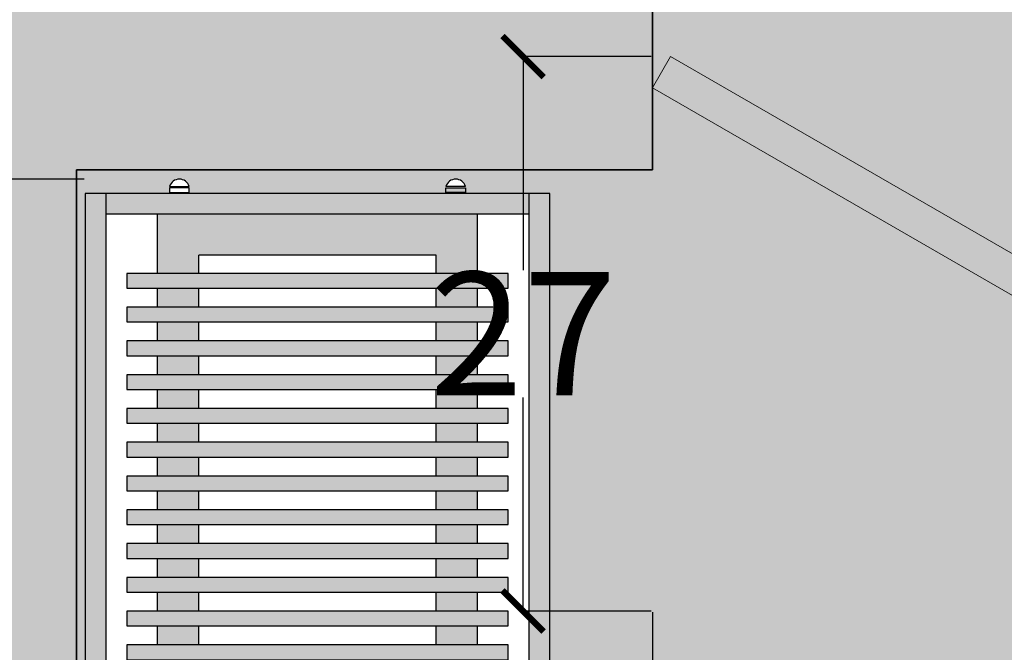
# Model space of a CAD drawing. Units: inches. Extents: x 1704 to 6393, y -157 to 1172.
# Tile 31 of 122: x 2351 to 2398, y 341 to 372. Entities that reach past the tile are written whole.
import ezdxf

# ---------------------------------------------------------------- set-up
doc = ezdxf.new("R2010")
doc.units = ezdxf.units.IN
doc.header["$MEASUREMENT"] = 0
for name, color, linetype, lineweight in [('A-ANNO-DIMS', 7, 'Continuous', 13), ('A-FURN', 8, 'Continuous', 18), ('A-WALL-PATT', 7, 'Continuous', 13), ('DOORS', 160, 'Continuous', 18), ('estofado', 7, 'Continuous', 25), ('WALLS', 7, 'Continuous', 35)]:
    doc.layers.add(name, color=color, linetype=linetype, lineweight=lineweight)
doc.layers.add('A-FLOR-PATT', color=7, linetype='Continuous', lineweight=13, true_color=0xf2f2f2)
doc.layers.add('MOBIL', color=7, linetype='Continuous')
doc.styles.get("Standard").update_dxf_attribs({"font": 'arial.ttf'})
doc.dimstyles.get("Standard").update_dxf_attribs({"dimtxt": 6, "dimasz": 2, "dimexe": 0.18, "dimexo": 0.0625, "dimgap": 0.09, "dimtad": 0, "dimtih": 1, "dimtoh": 1, "dimdec": 1, "dimzin": 0, "dimdsep": 46, "dimlunit": 3, "dimtxsty": 'Standard', "dimblk": 'ARCHTICK', "dimcen": 0.09, "dimadec": 0, "dimazin": 0, "dimtfac": 1, "dimtdec": 1, "dimtofl": 0, "dimtmove": 0, "dimatfit": 3, "dimfxl": 1, "dimtolj": 1, "dimtzin": 0, "dimarcsym": 0})

# ---------------------------------------------------------------- blocks, each defined once
blk = doc.blocks.new('Door - Left Hung 36 in.')
blk.add_lwpolyline([(0.75, -1.299), (0, 0), (31.177, 18), (31.927, 16.701)], close=True)
blk.add_arc((0, 0), 36, 0, 37.3101)
blk = doc.blocks.new('Aparador Aido WV')
at = {"layer": 'MOBIL'}
h = blk.add_hatch(color=256, dxfattribs=at)
h.set_gradient(color1=(226, 228, 228), one_color=1, tint=1, name='CYLINDER')
h.paths.add_polyline_path([(0.9, -0.02), (0.9, 0), (-0.9, 0), (-0.9, -0.02)])
h = blk.add_hatch(color=256, dxfattribs=at)
h.set_gradient(color1=(226, 228, 228), one_color=1, tint=1)
h.paths.add_polyline_path([(0.9, -0.02), (0.88, -0.02), (0.88, -0.43), (0.9, -0.43)])
h = blk.add_hatch(color=256, dxfattribs=at)
h.set_gradient(color1=(106, 79, 62), color2=(55, 41, 32), one_color=1, tint=0.17)
h.paths.add_polyline_path([(0.44785, -0.04017), (0.44785, -0.40983), (0.46222, -0.40983), (0.46222, -0.04017)])
h = blk.add_hatch(color=256, dxfattribs=at)
h.set_gradient(color1=(106, 79, 62), color2=(55, 41, 32), one_color=1, tint=0.17)
h.paths.add_polyline_path([(0.4806, -0.04017), (0.4806, -0.40983), (0.49497, -0.40983), (0.49497, -0.04017)])
h = blk.add_hatch(color=256, dxfattribs=at)
h.set_gradient(color1=(106, 79, 62), color2=(55, 41, 32), one_color=1, tint=0.17)
h.paths.add_polyline_path([(0.51335, -0.04017), (0.51335, -0.40983), (0.52772, -0.40983), (0.52772, -0.04017)])
h = blk.add_hatch(color=256, dxfattribs=at)
h.set_gradient(color1=(106, 79, 62), color2=(55, 41, 32), one_color=1, tint=0.17)
h.paths.add_polyline_path([(0.54611, -0.04017), (0.54611, -0.40983), (0.56047, -0.40983), (0.56047, -0.04017)])
h = blk.add_hatch(color=256, dxfattribs=at)
h.set_gradient(color1=(106, 79, 62), color2=(55, 41, 32), one_color=1, tint=0.17)
h.paths.add_polyline_path([(0.57886, -0.04017), (0.57886, -0.40983), (0.59322, -0.40983), (0.59322, -0.04017)])
h = blk.add_hatch(color=256, dxfattribs=at)
h.set_gradient(color1=(106, 79, 62), color2=(55, 41, 32), one_color=1, tint=0.17)
h.paths.add_polyline_path([(0.61161, -0.04017), (0.61161, -0.40983), (0.62597, -0.40983), (0.62597, -0.04017)])
h = blk.add_hatch(color=256, dxfattribs=at)
h.set_gradient(color1=(106, 79, 62), color2=(55, 41, 32), one_color=1, tint=0.17)
h.paths.add_polyline_path([(0.64436, -0.04017), (0.64436, -0.40983), (0.65873, -0.40983), (0.65873, -0.04017)])
h = blk.add_hatch(color=256, dxfattribs=at)
h.set_gradient(color1=(106, 79, 62), color2=(55, 41, 32), one_color=1, tint=0.17)
h.paths.add_polyline_path([(0.67711, -0.04017), (0.67711, -0.40983), (0.69148, -0.40983), (0.69148, -0.04017)])
h = blk.add_hatch(color=256, dxfattribs=at)
h.set_gradient(color1=(106, 79, 62), color2=(55, 41, 32), one_color=1, tint=0.17)
h.paths.add_polyline_path([(0.70986, -0.04017), (0.70986, -0.40983), (0.72423, -0.40983), (0.72423, -0.04017)])
h = blk.add_hatch(color=256, dxfattribs=at)
h.set_gradient(color1=(106, 79, 62), color2=(55, 41, 32), one_color=1, tint=0.17)
h.paths.add_polyline_path([(0.74262, -0.04017), (0.74262, -0.40983), (0.75698, -0.40983), (0.75698, -0.04017)])
h = blk.add_hatch(color=256, dxfattribs=at)
h.set_gradient(color1=(106, 79, 62), color2=(55, 41, 32), one_color=1, tint=0.17)
h.paths.add_polyline_path([(0.77537, -0.04017), (0.77537, -0.40983), (0.78973, -0.40983), (0.78973, -0.04017)])
h = blk.add_hatch(color=256, dxfattribs=at)
h.set_gradient(color1=(106, 79, 62), color2=(55, 41, 32), one_color=1, tint=0.17)
h.paths.add_polyline_path([(0.80812, -0.04017), (0.80812, -0.40983), (0.82248, -0.40983), (0.82248, -0.04017)])
h = blk.add_hatch(color=256, dxfattribs=at)
h.set_gradient(color1=(106, 79, 62), color2=(157, 117, 92), one_color=1, tint=0.49)
h.paths.add_polyline_path([(0.4806, -0.07), (0.46222, -0.07), (0.46222, -0.11), (0.4806, -0.11)])
h = blk.add_hatch(color=256, dxfattribs=at)
h.set_gradient(color1=(106, 79, 62), color2=(157, 117, 92), one_color=1, tint=0.49)
h.paths.add_polyline_path([(0.51335, -0.07), (0.49497, -0.07), (0.49497, -0.11), (0.51335, -0.11)])
h = blk.add_hatch(color=256, dxfattribs=at)
h.set_gradient(color1=(106, 79, 62), color2=(157, 117, 92), one_color=1, tint=0.49)
h.paths.add_polyline_path([(0.52772, -0.11), (0.54611, -0.11), (0.54611, -0.07), (0.52772, -0.07)])
h = blk.add_hatch(color=256, dxfattribs=at)
h.set_gradient(color1=(106, 79, 62), color2=(157, 117, 92), one_color=1, tint=0.49)
h.paths.add_polyline_path([(0.57886, -0.07), (0.56047, -0.07), (0.56047, -0.11), (0.57886, -0.11)])
h = blk.add_hatch(color=256, dxfattribs=at)
h.set_gradient(color1=(106, 79, 62), color2=(157, 117, 92), one_color=1, tint=0.49)
h.paths.add_polyline_path([(0.61161, -0.07), (0.59322, -0.07), (0.59322, -0.11), (0.61161, -0.11)])
h = blk.add_hatch(color=256, dxfattribs=at)
h.set_gradient(color1=(106, 79, 62), color2=(157, 117, 92), one_color=1, tint=0.49)
h.paths.add_polyline_path([(0.64436, -0.07), (0.62597, -0.07), (0.62597, -0.11), (0.64436, -0.11)])
h = blk.add_hatch(color=256, dxfattribs=at)
h.set_gradient(color1=(106, 79, 62), color2=(157, 117, 92), one_color=1, tint=0.49)
h.paths.add_polyline_path([(0.67711, -0.07), (0.65873, -0.07), (0.65873, -0.11), (0.67711, -0.11)])
h = blk.add_hatch(color=256, dxfattribs=at)
h.set_gradient(color1=(106, 79, 62), color2=(157, 117, 92), one_color=1, tint=0.49)
h.paths.add_polyline_path([(0.70986, -0.07), (0.69148, -0.07), (0.69148, -0.11), (0.70986, -0.11)])
h = blk.add_hatch(color=256, dxfattribs=at)
h.set_gradient(color1=(106, 79, 62), color2=(157, 117, 92), one_color=1, tint=0.49)
h.paths.add_polyline_path([(0.74262, -0.07), (0.72423, -0.07), (0.72423, -0.11), (0.74262, -0.11)])
h = blk.add_hatch(color=256, dxfattribs=at)
h.set_gradient(color1=(106, 79, 62), color2=(157, 117, 92), one_color=1, tint=0.49)
h.paths.add_polyline_path([(0.77537, -0.07), (0.75698, -0.07), (0.75698, -0.11), (0.77537, -0.11)])
h = blk.add_hatch(color=256, dxfattribs=at)
h.set_gradient(color1=(106, 79, 62), color2=(157, 117, 92), one_color=1, tint=0.49)
h.paths.add_polyline_path([(0.80812, -0.07), (0.78973, -0.07), (0.78973, -0.11), (0.80812, -0.11)])
h = blk.add_hatch(color=256, dxfattribs=at)
h.set_gradient(color1=(106, 79, 62), color2=(157, 117, 92), one_color=1, tint=0.49)
h.paths.add_polyline_path([(0.88, -0.07), (0.82248, -0.07), (0.82248, -0.11), (0.84, -0.11), (0.84, -0.34), (0.82248, -0.34), (0.82248, -0.38), (0.88, -0.38)])
h = blk.add_hatch(color=256, dxfattribs=at)
h.set_gradient(color1=(106, 79, 62), color2=(157, 117, 92), one_color=1, tint=0.49)
h.paths.add_polyline_path([(0.4806, -0.34), (0.46222, -0.34), (0.46222, -0.38), (0.4806, -0.38)])
h = blk.add_hatch(color=256, dxfattribs=at)
h.set_gradient(color1=(106, 79, 62), color2=(157, 117, 92), one_color=1, tint=0.49)
h.paths.add_polyline_path([(0.51335, -0.34), (0.49497, -0.34), (0.49497, -0.38), (0.51335, -0.38)])
h = blk.add_hatch(color=256, dxfattribs=at)
h.set_gradient(color1=(106, 79, 62), color2=(157, 117, 92), one_color=1, tint=0.49)
h.paths.add_polyline_path([(0.54611, -0.34), (0.52772, -0.34), (0.52772, -0.38), (0.54611, -0.38)])
h = blk.add_hatch(color=256, dxfattribs=at)
h.set_gradient(color1=(106, 79, 62), color2=(157, 117, 92), one_color=1, tint=0.49)
h.paths.add_polyline_path([(0.57886, -0.34), (0.56047, -0.34), (0.56047, -0.38), (0.57886, -0.38)])
h = blk.add_hatch(color=256, dxfattribs=at)
h.set_gradient(color1=(106, 79, 62), color2=(157, 117, 92), one_color=1, tint=0.49)
h.paths.add_polyline_path([(0.61161, -0.34), (0.59322, -0.34), (0.59322, -0.38), (0.61161, -0.38)])
h = blk.add_hatch(color=256, dxfattribs=at)
h.set_gradient(color1=(106, 79, 62), color2=(157, 117, 92), one_color=1, tint=0.49)
h.paths.add_polyline_path([(0.64436, -0.34), (0.62597, -0.34), (0.62597, -0.38), (0.64436, -0.38)])
h = blk.add_hatch(color=256, dxfattribs=at)
h.set_gradient(color1=(106, 79, 62), color2=(157, 117, 92), one_color=1, tint=0.49)
h.paths.add_polyline_path([(0.67711, -0.34), (0.65873, -0.34), (0.65873, -0.38), (0.67711, -0.38)])
h = blk.add_hatch(color=256, dxfattribs=at)
h.set_gradient(color1=(106, 79, 62), color2=(157, 117, 92), one_color=1, tint=0.49)
h.paths.add_polyline_path([(0.70986, -0.34), (0.69148, -0.34), (0.69148, -0.38), (0.70986, -0.38)])
h = blk.add_hatch(color=256, dxfattribs=at)
h.set_gradient(color1=(106, 79, 62), color2=(157, 117, 92), one_color=1, tint=0.49)
h.paths.add_polyline_path([(0.74262, -0.34), (0.72423, -0.34), (0.72423, -0.38), (0.74262, -0.38)])
h = blk.add_hatch(color=256, dxfattribs=at)
h.set_gradient(color1=(106, 79, 62), color2=(157, 117, 92), one_color=1, tint=0.49)
h.paths.add_polyline_path([(0.77537, -0.34), (0.75698, -0.34), (0.75698, -0.38), (0.77537, -0.38)])
h = blk.add_hatch(color=256, dxfattribs=at)
h.set_gradient(color1=(106, 79, 62), color2=(157, 117, 92), one_color=1, tint=0.49)
h.paths.add_polyline_path([(0.80812, -0.34), (0.78973, -0.34), (0.78973, -0.38), (0.80812, -0.38)])
h = blk.add_hatch(color=256, dxfattribs=at)
h.set_gradient(color1=(226, 228, 228), one_color=1, tint=1, name='CYLINDER')
h.paths.add_polyline_path([(0.9, -0.45), (0.9, -0.43), (-0.9, -0.43), (-0.9, -0.45)])
at = {"layer": 'estofado', "ltscale": 0.5}
for p, q in [((0.46222, -0.07), (0.4806, -0.07)), ((0.49497, -0.07), (0.51335, -0.07)), ((0.52772, -0.07), (0.54611, -0.07)), ((0.56047, -0.07), (0.57886, -0.07)), ((0.59322, -0.07), (0.61161, -0.07)), ((0.62597, -0.07), (0.64436, -0.07)), ((0.65873, -0.07), (0.67711, -0.07)), ((0.69148, -0.07), (0.70986, -0.07)), ((0.72423, -0.07), (0.74262, -0.07)), ((0.75698, -0.07), (0.77537, -0.07)), ((0.78973, -0.07), (0.80812, -0.07)), ((0.82248, -0.07), (0.88, -0.07)), ((0.90671, -0.0817), (0.90671, -0.10055)), ((0.46222, -0.11), (0.4806, -0.11)), ((0.49497, -0.11), (0.51335, -0.11)), ((0.52772, -0.11), (0.54611, -0.11)), ((0.56047, -0.11), (0.57886, -0.11)), ((0.59322, -0.11), (0.61161, -0.11)), ((0.62597, -0.11), (0.64436, -0.11)), ((0.65873, -0.11), (0.67711, -0.11)), ((0.69148, -0.11), (0.70986, -0.11)), ((0.72423, -0.11), (0.74262, -0.11)), ((0.75698, -0.11), (0.77537, -0.11)), ((0.78973, -0.11), (0.80812, -0.11)), ((0.82248, -0.11), (0.84, -0.11)), ((0.84, -0.34), (0.84, -0.11)), ((0.46222, -0.34), (0.4806, -0.34)), ((0.49497, -0.34), (0.51335, -0.34)), ((0.52772, -0.34), (0.54611, -0.34)), ((0.56047, -0.34), (0.57886, -0.34)), ((0.59322, -0.34), (0.61161, -0.34)), ((0.62597, -0.34), (0.64436, -0.34)), ((0.65873, -0.34), (0.67711, -0.34)), ((0.69148, -0.34), (0.70986, -0.34)), ((0.72423, -0.34), (0.74262, -0.34)), ((0.75698, -0.34), (0.77537, -0.34)), ((0.78973, -0.34), (0.80812, -0.34)), ((0.82248, -0.34), (0.84, -0.34)), ((0.90671, -0.3683), (0.90671, -0.34945)), ((0.46222, -0.38), (0.4806, -0.38)), ((0.49497, -0.38), (0.51335, -0.38)), ((0.52772, -0.38), (0.54611, -0.38)), ((0.56047, -0.38), (0.57886, -0.38)), ((0.59322, -0.38), (0.61161, -0.38)), ((0.62597, -0.38), (0.64436, -0.38)), ((0.65873, -0.38), (0.67711, -0.38)), ((0.69148, -0.38), (0.70986, -0.38)), ((0.72423, -0.38), (0.74262, -0.38)), ((0.75698, -0.38), (0.77537, -0.38)), ((0.78973, -0.38), (0.80812, -0.38)), ((0.82248, -0.38), (0.88, -0.38))]:
    blk.add_line(p, q, dxfattribs=at)
for points in [[(0.44785, -0.04017), (0.44785, -0.40983), (0.46222, -0.40983), (0.46222, -0.04017)], [(0.4806, -0.04017), (0.4806, -0.40983), (0.49497, -0.40983), (0.49497, -0.04017)], [(0.51335, -0.04017), (0.51335, -0.40983), (0.52772, -0.40983), (0.52772, -0.04017)], [(0.54611, -0.04017), (0.54611, -0.40983), (0.56047, -0.40983), (0.56047, -0.04017)], [(0.57886, -0.04017), (0.57886, -0.40983), (0.59322, -0.40983), (0.59322, -0.04017)], [(0.61161, -0.04017), (0.61161, -0.40983), (0.62597, -0.40983), (0.62597, -0.04017)], [(0.64436, -0.04017), (0.64436, -0.40983), (0.65873, -0.40983), (0.65873, -0.04017)], [(0.67711, -0.04017), (0.67711, -0.40983), (0.69148, -0.40983), (0.69148, -0.04017)], [(0.70986, -0.04017), (0.70986, -0.40983), (0.72423, -0.40983), (0.72423, -0.04017)], [(0.74262, -0.04017), (0.74262, -0.40983), (0.75698, -0.40983), (0.75698, -0.04017)], [(0.77537, -0.04017), (0.77537, -0.40983), (0.78973, -0.40983), (0.78973, -0.04017)], [(0.80812, -0.04017), (0.80812, -0.40983), (0.82248, -0.40983), (0.82248, -0.04017)], [(0.90536, -0.0817), (0.90086, -0.0817), (0.90086, -0.10055), (0.90536, -0.10055)], [(0.90536, -0.3683), (0.90086, -0.3683), (0.90086, -0.34945), (0.90536, -0.34945)]]:
    blk.add_lwpolyline(points, close=True, dxfattribs=at)
for centre in [(0.90401, -0.09113), (0.90401, -0.35887)]:
    blk.add_arc(centre, 0.0098, 285.98491, 74.01509, dxfattribs=at)
at = {"layer": 'MOBIL'}
for p, q in [((0.9, -0.02), (-0.9, -0.02)), ((0.88, -0.43), (0.88, -0.02)), ((-0.9, -0.43), (0.9, -0.43))]:
    blk.add_line(p, q, dxfattribs=at)
blk.add_lwpolyline([(-0.9, -0.45), (0.9, -0.45), (0.9, 0), (-0.9, 0)], close=True, dxfattribs=at)
blk = doc.blocks.new('_ArchTick')
at = {"color": 0, "linetype": 'ByBlock', "const_width": 0.15}
blk.add_lwpolyline([(-0.5, -0.5), (0.5, 0.5)], dxfattribs=at)
blk = doc.blocks.new('*D30')
at = {"layer": 'A-ANNO-DIMS', "color": 0, "lineweight": -2, "transparency": 16777216}
for p, q in [((2381.349, 342.693), (2381.349, 336.276)), ((2423.349, 342.693), (2423.349, 336.276)), ((2381.349, 336.456), (2384.404, 336.456)), ((2423.349, 336.456), (2420.293, 336.456))]:
    blk.add_line(p, q, dxfattribs=at)
at = {"layer": 'Defpoints', "color": 0, "lineweight": -3, "transparency": 16777216}
for p in [(2381.349, 342.756), (2423.349, 342.756), (2423.349, 336.456)]:
    blk.add_point(p, dxfattribs=at)
at = {"layer": 'A-ANNO-DIMS', "color": 0, "lineweight": -2, "transparency": 16777216, "xscale": 2, "yscale": 2, "zscale": 2, "rotation": 180}
blk.add_blockref('_ArchTick', (2381.349, 336.456), dxfattribs=at)
at = {"layer": 'A-ANNO-DIMS', "color": 0, "lineweight": -2, "transparency": 16777216, "xscale": 2, "yscale": 2, "zscale": 2}
blk.add_blockref('_ArchTick', (2423.349, 336.456), dxfattribs=at)
at = {"layer": 'A-ANNO-DIMS', "color": 0, "transparency": 16777216, "insert": (2402.349, 336.456), "char_height": 6, "attachment_point": 5}
blk.add_mtext('\\A1;DOOR 42', dxfattribs=at)
blk = doc.blocks.new('*D31')
at = {"layer": 'A-ANNO-DIMS', "color": 0, "lineweight": -2, "transparency": 16777216}
for p, q in [((2381.286, 369.729), (2374.869, 369.729)), ((2375.049, 369.729), (2375.049, 359.344)), ((2375.049, 342.756), (2375.049, 353.14)), ((2381.286, 342.756), (2374.869, 342.756))]:
    blk.add_line(p, q, dxfattribs=at)
at = {"layer": 'Defpoints', "color": 0, "lineweight": -3, "transparency": 16777216}
for p in [(2381.349, 369.729), (2375.049, 342.756), (2381.349, 342.756)]:
    blk.add_point(p, dxfattribs=at)
at = {"layer": 'A-ANNO-DIMS', "color": 0, "lineweight": -2, "transparency": 16777216, "xscale": 2, "yscale": 2, "zscale": 2}
for p, rotation in [((2375.049, 369.729), 90), ((2375.049, 342.756), 270)]:
    blk.add_blockref('_ArchTick', p, dxfattribs=dict(at, rotation=rotation))
at = {"layer": 'A-ANNO-DIMS', "color": 0, "transparency": 16777216, "insert": (2375.049, 356.242), "char_height": 6, "attachment_point": 5}
blk.add_mtext('\\A1;27', dxfattribs=at)
blk = doc.blocks.new('*D68')
at = {"layer": 'A-ANNO-DIMS', "color": 0, "lineweight": -2, "transparency": 16777216}
for p, q in [((2353.706, 363.767), (2339.834, 363.767)), ((2340.014, 363.767), (2340.014, 321.111)), ((2340.014, 272.066), (2340.014, 314.722)), ((2353.706, 272.066), (2339.834, 272.066))]:
    blk.add_line(p, q, dxfattribs=at)
at = {"layer": 'Defpoints', "color": 0, "lineweight": -3, "transparency": 16777216}
for p in [(2340.014, 363.767), (2353.769, 363.767), (2353.769, 272.066)]:
    blk.add_point(p, dxfattribs=at)
at = {"layer": 'A-ANNO-DIMS', "color": 0, "lineweight": -2, "transparency": 16777216, "xscale": 2, "yscale": 2, "zscale": 2}
for p, rotation in [((2340.014, 363.767), 90), ((2340.014, 272.066), 270)]:
    blk.add_blockref('_ArchTick', p, dxfattribs=dict(at, rotation=rotation))
at = {"layer": 'A-ANNO-DIMS', "color": 0, "transparency": 16777216, "insert": (2340.014, 317.916), "char_height": 6, "attachment_point": 5}
blk.add_mtext('\\A1;SIDEBOARD 92', dxfattribs=at)
blk = doc.blocks.new('*D93')
at = {"layer": 'A-ANNO-DIMS', "color": 0, "lineweight": -2, "transparency": 16777216}
for p, q in [((2605.286, 895.213), (1829.698, 895.213)), ((1829.878, 895.213), (1829.878, 495.866)), ((1829.878, 90.213), (1829.878, 489.56)), ((2605.286, 90.213), (1829.698, 90.213))]:
    blk.add_line(p, q, dxfattribs=at)
at = {"layer": 'Defpoints', "color": 0, "lineweight": -3, "transparency": 16777216}
for p in [(2605.349, 895.213), (1829.878, 90.213), (2605.349, 90.213)]:
    blk.add_point(p, dxfattribs=at)
at = {"layer": 'A-ANNO-DIMS', "color": 0, "lineweight": -2, "transparency": 16777216, "xscale": 2, "yscale": 2, "zscale": 2}
for p, rotation in [((1829.878, 895.213), 90), ((1829.878, 90.213), 270)]:
    blk.add_blockref('_ArchTick', p, dxfattribs=dict(at, rotation=rotation))
at = {"layer": 'A-ANNO-DIMS', "color": 0, "transparency": 16777216, "insert": (1829.878, 492.713), "char_height": 6, "attachment_point": 5}
blk.add_mtext('\\A1;805', dxfattribs=at)

msp = doc.modelspace()

# ---------------------------------------------------------------- hatches: boundary and pattern name
at = {"layer": 'A-FLOR-PATT', "transparency": 33554528}
h = msp.add_hatch(color=256, dxfattribs=at)
h.dxf.hatch_style = 1
h.paths.add_polyline_path([(2325.349, 863.213), (2325.349, 887.213), (2263.349, 887.213), (2167.349, 887.213), (2081.349, 887.213), (2081.349, 719.213), (2277.349, 719.213), (2277.349, 711.213), (2277.349, 372.213), (2349.349, 372.213), (2381.349, 372.213), (2381.349, 364.213), (2353.349, 364.213), (2353.349, 270.213), (2381.349, 270.213), (2381.349, 266.213), (2357.349, 266.213), (2357.349, 98.213), (2381.349, 98.213), (2385.181, 98.213), (2386.482, 98.213), (2424.215, 98.213), (2425.516, 98.213), (2429.349, 98.213), (2597.349, 98.213), (2597.349, 146.213), (2597.349, 218.213), (2597.349, 266.213), (2423.349, 266.213), (2423.349, 270.213), (2473.349, 270.213), (2473.349, 294.213), (2477.349, 294.213), (2477.349, 270.213), (2547.349, 270.213), (2547.349, 364.213), (2477.349, 364.213), (2477.349, 318.213), (2473.349, 318.213), (2473.349, 364.213), (2423.349, 364.213), (2423.349, 372.213), (2469.349, 372.213), (2469.349, 459.213), (2469.349, 538.213), (2350.349, 538.213), (2350.349, 565.713), (2358.349, 565.713), (2358.349, 545.213), (2420.349, 545.213), (2420.349, 610.213), (2358.349, 610.213), (2358.349, 589.713), (2350.349, 589.713), (2350.349, 615.213), (2425.349, 615.213), (2425.349, 607.213), (2425.349, 546.213), (2469.349, 546.213), (2514.349, 546.213), (2514.349, 607.213), (2449.349, 607.213), (2449.349, 615.213), (2451.738, 615.213), (2451.738, 659.213), (2427.738, 659.213), (2427.738, 665.213), (2367.738, 665.213), (2367.738, 667.213), (2367.738, 711.213), (2325.349, 711.213), (2325.349, 719.213), (2325.349, 755.213), (2325.349, 763.213)])
h.paths.add_polyline_path([(2233.858, 822.533, -0.187247), (2233.858, 809.14), (2231.697, 808.804, 0.084893), (2233.131, 814.486), (2230.424, 814.486, -0.104258), (2228.553, 808.313), (2217.751, 807.156, -0.222222), (2217.751, 824.517), (2228.553, 823.359, -0.104258), (2230.424, 817.186), (2233.131, 817.186, 0.084893), (2231.697, 822.868)], flags=16)
h.paths.add_polyline_path([(2213.621, 833.197), (2213.621, 798.475), (2156.048, 798.475), (2156.048, 833.197)], flags=16)
h.paths.add_polyline_path([(2203.932, 848.099), (2205.089, 837.296, -0.222222), (2187.728, 837.296), (2188.885, 848.099, -0.104258), (2195.058, 849.969), (2195.058, 852.676, 0.084893), (2189.377, 851.242), (2189.712, 853.404, -0.187247), (2203.105, 853.404), (2203.44, 851.242, 0.084893), (2197.759, 852.676), (2197.759, 849.969, -0.104258)], flags=16)
h.paths.add_polyline_path([(2181.941, 837.296, -0.222222), (2164.58, 837.296), (2165.737, 848.099, -0.104258), (2171.91, 849.969), (2171.91, 852.676, 0.084893), (2166.229, 851.242), (2166.564, 853.404, -0.187247), (2179.957, 853.404), (2180.292, 851.242, 0.084893), (2174.611, 852.676), (2174.611, 849.969, -0.104258), (2180.784, 848.099)], flags=16)
h.paths.add_polyline_path([(2205.089, 794.376), (2203.932, 783.574, -0.104258), (2197.759, 781.703), (2197.759, 778.996, 0.084893), (2203.44, 780.43), (2203.105, 778.269, -0.187247), (2189.712, 778.269), (2189.377, 780.43, 0.084893), (2195.058, 778.996), (2195.058, 781.703, -0.104258), (2188.885, 783.574), (2187.728, 794.376, -0.222222)], flags=16)
h.paths.add_polyline_path([(2181.941, 794.376), (2180.784, 783.574, -0.104258), (2174.611, 781.703), (2174.611, 778.996, 0.084893), (2180.292, 780.43), (2179.957, 778.269, -0.187247), (2166.564, 778.269), (2166.229, 780.43, 0.084893), (2171.91, 778.996), (2171.91, 781.703, -0.104258), (2165.737, 783.574), (2164.58, 794.376, -0.222222)], flags=16)
h.paths.add_polyline_path([(2151.918, 807.156), (2141.116, 808.313, -0.104258), (2139.245, 814.486), (2136.539, 814.486, 0.084893), (2137.972, 808.804), (2135.811, 809.14, -0.187247), (2135.811, 822.533), (2137.972, 822.868, 0.084893), (2136.539, 817.186), (2139.245, 817.186, -0.104258), (2141.116, 823.359), (2151.918, 824.517, -0.222222)], flags=16)
h.paths.add_polyline_path([(2357.868, 363.41), (2358.814, 363.41, 0.75376)], flags=16)
h.paths.add_polyline_path([(2372.241, 363.117), (2372.248, 363.117), (2372.248, 363.343), (2371.302, 363.343), (2371.302, 363.139, -1.360391)], flags=16)
h.paths.add_polyline_path([(2371.309, 272.716), (2371.302, 272.716), (2371.302, 272.49), (2372.248, 272.49), (2372.248, 272.693, -1.360391)], flags=16)
h.paths.add_polyline_path([(2357.875, 272.716), (2357.868, 272.716), (2357.868, 272.49), (2358.814, 272.49), (2358.814, 272.693, -1.360391)], flags=16)
h.paths.add_polyline_path([(2353.769, 363.074), (2376.347, 363.074), (2376.347, 272.759), (2353.769, 272.759)], flags=16)
h.paths.add_polyline_path([(2354.772, 362.07), (2375.344, 362.07), (2375.344, 273.762), (2354.772, 273.762)], flags=0)
h.paths.add_polyline_path([(2357.868, 363.343), (2358.814, 363.343), (2358.814, 363.117), (2357.868, 363.117)], flags=16)
h.paths.add_polyline_path([(2359.288, 359.184), (2359.288, 360.063), (2370.828, 360.063), (2370.828, 359.184), (2374.332, 359.184), (2374.332, 358.464), (2372.835, 358.464), (2372.835, 357.541), (2374.332, 357.541), (2374.332, 356.82), (2372.835, 356.82), (2372.835, 355.898), (2374.332, 355.898), (2374.332, 355.177), (2372.835, 355.177), (2372.835, 354.254), (2374.332, 354.254), (2374.332, 353.534), (2372.835, 353.534), (2372.835, 352.611), (2374.332, 352.611), (2374.332, 351.89), (2372.835, 351.89), (2372.835, 350.968), (2374.332, 350.968), (2374.332, 350.247), (2372.835, 350.247), (2372.835, 349.324), (2374.332, 349.324), (2374.332, 348.604), (2372.835, 348.604), (2372.835, 347.681), (2374.332, 347.681), (2374.332, 346.96), (2372.835, 346.96), (2372.835, 346.038), (2374.332, 346.038), (2374.332, 345.317), (2372.835, 345.317), (2372.835, 344.395), (2374.332, 344.395), (2374.332, 343.674), (2372.835, 343.674), (2372.835, 342.751), (2374.332, 342.751), (2374.332, 342.03), (2372.835, 342.03), (2372.835, 341.108), (2374.332, 341.108), (2374.332, 340.387), (2372.835, 340.387), (2372.835, 339.465), (2374.332, 339.465), (2374.332, 338.744), (2372.835, 338.744), (2372.835, 337.821), (2374.332, 337.821), (2374.332, 337.1), (2372.835, 337.1), (2372.835, 336.178), (2374.332, 336.178), (2374.332, 335.457), (2372.835, 335.457), (2372.835, 334.535), (2374.332, 334.535), (2374.332, 333.814), (2372.835, 333.814), (2372.835, 332.891), (2374.332, 332.891), (2374.332, 332.171), (2372.835, 332.171), (2372.835, 331.248), (2374.332, 331.248), (2374.332, 330.527), (2372.835, 330.527), (2372.835, 329.605), (2374.332, 329.605), (2374.332, 328.884), (2372.835, 328.884), (2372.835, 327.961), (2374.332, 327.961), (2374.332, 327.241), (2372.835, 327.241), (2372.835, 326.318), (2374.332, 326.318), (2374.332, 325.597), (2372.835, 325.597), (2372.835, 324.675), (2374.332, 324.675), (2374.332, 323.954), (2372.835, 323.954), (2372.835, 323.031), (2374.332, 323.031), (2374.332, 322.311), (2372.835, 322.311), (2372.835, 321.388), (2374.332, 321.388), (2374.332, 320.667), (2372.835, 320.667), (2372.835, 319.745), (2374.332, 319.745), (2374.332, 319.024), (2372.835, 319.024), (2372.835, 318.102), (2374.332, 318.102), (2374.332, 317.381), (2372.835, 317.381), (2372.835, 316.458), (2374.332, 316.458), (2374.332, 315.737), (2372.835, 315.737), (2372.835, 314.815), (2374.332, 314.815), (2374.332, 314.094), (2372.835, 314.094), (2372.835, 313.172), (2374.332, 313.172), (2374.332, 312.451), (2372.835, 312.451), (2372.835, 311.528), (2374.332, 311.528), (2374.332, 310.807), (2372.835, 310.807), (2372.835, 309.885), (2374.332, 309.885), (2374.332, 309.164), (2372.835, 309.164), (2372.835, 308.242), (2374.332, 308.242), (2374.332, 307.521), (2372.835, 307.521), (2372.835, 306.598), (2374.332, 306.598), (2374.332, 305.878), (2372.835, 305.878), (2372.835, 304.955), (2374.332, 304.955), (2374.332, 304.234), (2372.835, 304.234), (2372.835, 303.312), (2374.332, 303.312), (2374.332, 302.591), (2372.835, 302.591), (2372.835, 301.668), (2374.332, 301.668), (2374.332, 300.948), (2372.835, 300.948), (2372.835, 300.025), (2374.332, 300.025), (2374.332, 299.304), (2372.835, 299.304), (2372.835, 298.382), (2374.332, 298.382), (2374.332, 297.661), (2372.835, 297.661), (2372.835, 296.738), (2374.332, 296.738), (2374.332, 296.018), (2372.835, 296.018), (2372.835, 295.095), (2374.332, 295.095), (2374.332, 294.374), (2372.835, 294.374), (2372.835, 293.452), (2374.332, 293.452), (2374.332, 292.731), (2372.835, 292.731), (2372.835, 291.809), (2374.332, 291.809), (2374.332, 291.088), (2372.835, 291.088), (2372.835, 290.165), (2374.332, 290.165), (2374.332, 289.444), (2372.835, 289.444), (2372.835, 288.522), (2374.332, 288.522), (2374.332, 287.801), (2372.835, 287.801), (2372.835, 286.879), (2374.332, 286.879), (2374.332, 286.158), (2372.835, 286.158), (2372.835, 285.235), (2374.332, 285.235), (2374.332, 284.514), (2372.835, 284.514), (2372.835, 283.592), (2374.332, 283.592), (2374.332, 282.871), (2372.835, 282.871), (2372.835, 281.949), (2374.332, 281.949), (2374.332, 281.228), (2372.835, 281.228), (2372.835, 280.305), (2374.332, 280.305), (2374.332, 279.585), (2372.835, 279.585), (2372.835, 278.662), (2374.332, 278.662), (2374.332, 277.941), (2372.835, 277.941), (2372.835, 277.019), (2374.332, 277.019), (2374.332, 276.298), (2370.828, 276.298), (2370.828, 275.769), (2359.288, 275.769), (2359.288, 276.298), (2355.784, 276.298), (2355.784, 277.019), (2357.281, 277.019), (2357.281, 277.941), (2355.784, 277.941), (2355.784, 278.662), (2357.281, 278.662), (2357.281, 279.585), (2355.784, 279.585), (2355.784, 280.305), (2357.281, 280.305), (2357.281, 281.228), (2355.784, 281.228), (2355.784, 281.949), (2357.281, 281.949), (2357.281, 282.871), (2355.784, 282.871), (2355.784, 283.592), (2357.281, 283.592), (2357.281, 284.514), (2355.784, 284.514), (2355.784, 285.235), (2357.281, 285.235), (2357.281, 286.158), (2355.784, 286.158), (2355.784, 286.879), (2357.281, 286.879), (2357.281, 287.801), (2355.784, 287.801), (2355.784, 288.522), (2357.281, 288.522), (2357.281, 289.444), (2355.784, 289.444), (2355.784, 290.165), (2357.281, 290.165), (2357.281, 291.088), (2355.784, 291.088), (2355.784, 291.809), (2357.281, 291.809), (2357.281, 292.731), (2355.784, 292.731), (2355.784, 293.452), (2357.281, 293.452), (2357.281, 294.374), (2355.784, 294.374), (2355.784, 295.095), (2357.281, 295.095), (2357.281, 296.018), (2355.784, 296.018), (2355.784, 296.738), (2357.281, 296.738), (2357.281, 297.661), (2355.784, 297.661), (2355.784, 298.382), (2357.281, 298.382), (2357.281, 299.304), (2355.784, 299.304), (2355.784, 300.025), (2357.281, 300.025), (2357.281, 300.948), (2355.784, 300.948), (2355.784, 301.668), (2357.281, 301.668), (2357.281, 302.591), (2355.784, 302.591), (2355.784, 303.312), (2357.281, 303.312), (2357.281, 304.234), (2355.784, 304.234), (2355.784, 304.955), (2357.281, 304.955), (2357.281, 305.878), (2355.784, 305.878), (2355.784, 306.598), (2357.281, 306.598), (2357.281, 307.521), (2355.784, 307.521), (2355.784, 308.242), (2357.281, 308.242), (2357.281, 309.164), (2355.784, 309.164), (2355.784, 309.885), (2357.281, 309.885), (2357.281, 310.807), (2355.784, 310.807), (2355.784, 311.528), (2357.281, 311.528), (2357.281, 312.451), (2355.784, 312.451), (2355.784, 313.172), (2357.281, 313.172), (2357.281, 314.094), (2355.784, 314.094), (2355.784, 314.815), (2357.281, 314.815), (2357.281, 315.737), (2355.784, 315.737), (2355.784, 316.458), (2357.281, 316.458), (2357.281, 317.381), (2355.784, 317.381), (2355.784, 318.102), (2357.281, 318.102), (2357.281, 319.024), (2355.784, 319.024), (2355.784, 319.745), (2357.281, 319.745), (2357.281, 320.667), (2355.784, 320.667), (2355.784, 321.388), (2357.281, 321.388), (2357.281, 322.311), (2355.784, 322.311), (2355.784, 323.031), (2357.281, 323.031), (2357.281, 323.954), (2355.784, 323.954), (2355.784, 324.675), (2357.281, 324.675), (2357.281, 325.597), (2355.784, 325.597), (2355.784, 326.318), (2357.281, 326.318), (2357.281, 327.241), (2355.784, 327.241), (2355.784, 327.961), (2357.281, 327.961), (2357.281, 328.884), (2355.784, 328.884), (2355.784, 329.605), (2357.281, 329.605), (2357.281, 330.527), (2355.784, 330.527), (2355.784, 331.248), (2357.281, 331.248), (2357.281, 332.171), (2355.784, 332.171), (2355.784, 332.891), (2357.281, 332.891), (2357.281, 333.814), (2355.784, 333.814), (2355.784, 334.535), (2357.281, 334.535), (2357.281, 335.457), (2355.784, 335.457), (2355.784, 336.178), (2357.281, 336.178), (2357.281, 337.1), (2355.784, 337.1), (2355.784, 337.821), (2357.281, 337.821), (2357.281, 338.744), (2355.784, 338.744), (2355.784, 339.465), (2357.281, 339.465), (2357.281, 340.387), (2355.784, 340.387), (2355.784, 341.108), (2357.281, 341.108), (2357.281, 342.03), (2355.784, 342.03), (2355.784, 342.751), (2357.281, 342.751), (2357.281, 343.674), (2355.784, 343.674), (2355.784, 344.395), (2357.281, 344.395), (2357.281, 345.317), (2355.784, 345.317), (2355.784, 346.038), (2357.281, 346.038), (2357.281, 346.96), (2355.784, 346.96), (2355.784, 347.681), (2357.281, 347.681), (2357.281, 348.604), (2355.784, 348.604), (2355.784, 349.324), (2357.281, 349.324), (2357.281, 350.247), (2355.784, 350.247), (2355.784, 350.968), (2357.281, 350.968), (2357.281, 351.89), (2355.784, 351.89), (2355.784, 352.611), (2357.281, 352.611), (2357.281, 353.534), (2355.784, 353.534), (2355.784, 354.254), (2357.281, 354.254), (2357.281, 355.177), (2355.784, 355.177), (2355.784, 355.898), (2357.281, 355.898), (2357.281, 356.82), (2355.784, 356.82), (2355.784, 357.541), (2357.281, 357.541), (2357.281, 358.464), (2355.784, 358.464), (2355.784, 359.184)], flags=0)
at = {"layer": 'A-WALL-PATT', "transparency": 33554643}
h = msp.add_hatch(color=256, dxfattribs=at)
h.dxf.hatch_style = 1
h.paths.add_polyline_path([(2167.349, 895.213), (2073.349, 895.213), (2073.349, 887.213), (2081.349, 887.213), (2167.349, 887.213)])
h.paths.add_polyline_path([(2465.349, 895.213), (2273.349, 895.213), (2273.349, 903.213), (2263.349, 903.213), (2263.349, 895.213), (2263.349, 887.213), (2325.349, 887.213), (2325.349, 863.213), (2333.349, 863.213), (2333.349, 887.213), (2465.349, 887.213)])
h.paths.add_polyline_path([(2533.349, 895.213), (2513.349, 895.213), (2513.349, 887.213), (2513.349, 861.213), (2517.349, 861.213), (2517.349, 887.213), (2533.349, 887.213)])
h.paths.add_polyline_path([(2605.349, 895.213), (2581.349, 895.213), (2581.349, 887.213), (2597.349, 887.213), (2597.349, 854.213), (2605.349, 854.213)])
h.paths.add_polyline_path([(2605.349, 752.213), (2629.349, 752.213), (2629.349, 716.213), (2605.349, 716.213), (2605.349, 712.213), (2719.349, 712.213), (2719.349, 716.213), (2631.349, 716.213), (2631.349, 754.213), (2605.349, 754.213), (2605.349, 794.213), (2597.349, 794.213), (2597.349, 787.213), (2517.349, 787.213), (2517.349, 813.213), (2513.349, 813.213), (2513.349, 783.213), (2517.349, 783.213), (2597.349, 783.213), (2597.349, 719.213), (2517.349, 719.213), (2517.349, 753.213), (2513.349, 753.213), (2513.349, 719.213), (2365.349, 719.213), (2365.349, 763.213), (2325.349, 763.213), (2325.349, 755.213), (2357.349, 755.213), (2357.349, 719.213), (2325.349, 719.213), (2325.349, 711.213), (2547.349, 711.213), (2547.349, 615.213), (2449.349, 615.213), (2449.349, 607.213), (2514.349, 607.213), (2514.349, 546.213), (2439.349, 546.213), (2425.349, 546.213), (2425.349, 607.213), (2425.349, 615.213), (2350.349, 615.213), (2350.349, 589.713), (2358.349, 589.713), (2358.349, 610.213), (2420.349, 610.213), (2420.349, 545.213), (2358.349, 545.213), (2358.349, 565.713), (2350.349, 565.713), (2350.349, 538.213), (2469.349, 538.213), (2469.349, 459.213), (2469.349, 372.213), (2423.349, 372.213), (2423.349, 364.213), (2473.349, 364.213), (2473.349, 318.213), (2477.349, 318.213), (2477.349, 364.213), (2547.349, 364.213), (2547.349, 352.213), (2549.349, 352.213), (2549.349, 364.213), (2597.349, 364.213), (2597.349, 328.213), (2549.349, 328.213), (2547.349, 328.213), (2547.349, 326.213), (2549.349, 326.213), (2597.349, 326.213), (2605.349, 326.213), (2605.349, 377.057), (2597.349, 377.057), (2597.349, 372.213), (2477.349, 372.213), (2477.349, 451.213), (2597.349, 451.213), (2605.349, 451.213), (2605.349, 459.213), (2597.349, 459.213), (2477.349, 459.213), (2477.349, 538.213), (2597.349, 538.213), (2597.349, 495.213), (2605.349, 495.213), (2605.349, 512.213), (2631.349, 512.213), (2631.349, 568.213), (2605.349, 568.213), (2605.349, 577.213), (2597.349, 577.213), (2597.349, 542.213), (2518.349, 542.213), (2518.349, 607.213), (2532.349, 607.213), (2605.349, 607.213), (2605.349, 615.213), (2597.349, 615.213), (2551.349, 615.213), (2551.349, 711.213), (2597.349, 711.213), (2597.349, 645.213), (2605.349, 645.213), (2605.349, 712.213), (2605.349, 716.213)])
h.paths.add_polyline_path([(2605.349, 566.213), (2629.349, 566.213), (2629.349, 514.213), (2605.349, 514.213)], flags=16)
h.paths.add_polyline_path([(2381.349, 372.213), (2349.349, 372.213), (2349.349, 202.213), (2337.349, 202.213), (2337.349, 194.213), (2349.349, 194.213), (2349.349, 90.213), (2349.349, 72.213), (2357.349, 72.213), (2357.349, 90.213), (2381.349, 90.213), (2381.349, 98.213), (2357.349, 98.213), (2357.349, 266.213), (2381.349, 266.213), (2381.349, 270.213), (2353.349, 270.213), (2353.349, 364.213), (2381.349, 364.213)])
h.paths.add_polyline_path([(2605.349, 302.213), (2597.349, 302.213), (2597.349, 270.213), (2477.349, 270.213), (2477.349, 294.213), (2473.349, 294.213), (2473.349, 270.213), (2423.349, 270.213), (2423.349, 266.213), (2597.349, 266.213), (2597.349, 218.213), (2605.349, 218.213)])
h.paths.add_polyline_path([(2605.349, 146.213), (2597.349, 146.213), (2597.349, 98.213), (2429.349, 98.213), (2429.349, 90.213), (2597.349, 90.213), (2597.349, 72.213), (2605.349, 72.213), (2605.349, 90.213)])
h.paths.add_polyline_path([(2225.349, 202.213), (2049.349, 202.213), (2049.349, 194.213), (2225.349, 194.213)])
h.paths.add_polyline_path([(2289.349, 202.213), (2277.349, 202.213), (2273.349, 202.213), (2269.516, 202.213), (2269.516, 194.213), (2273.349, 194.213), (2277.349, 194.213), (2289.349, 194.213)])
h.paths.add_polyline_path([(2273.349, 372.213), (2029.19, 372.213), (2029.19, 364.213), (2273.349, 364.213)])
h.paths.add_polyline_path([(2277.349, 545.213), (2213.349, 545.213), (2213.349, 573.213), (2205.349, 573.213), (2177.349, 573.213), (2177.349, 545.213), (2073.349, 545.213), (2073.349, 538.213), (2081.349, 538.213), (2277.349, 538.213)])
h.paths.add_polyline_path([(2181.349, 545.213), (2181.349, 569.213), (2205.349, 569.213), (2205.349, 545.213)], flags=16)
h.paths.add_polyline_path([(2277.349, 719.213), (2081.349, 719.213), (2073.349, 719.213), (2073.349, 711.213), (2154.575, 711.213), (2205.349, 711.213), (2205.349, 687.213), (2205.349, 629.213), (2213.349, 629.213), (2273.349, 629.213), (2273.349, 631.213), (2207.349, 631.213), (2207.349, 707.213), (2231.349, 707.213), (2231.349, 709.213), (2207.349, 709.213), (2207.349, 711.213), (2277.349, 711.213)])

# ---------------------------------------------------------------- linework, layer by layer
at = {"layer": 'WALLS'}
for p, q in [((2381.349, 364.213), (2381.349, 372.213)), ((2353.349, 270.213), (2353.349, 364.213)), ((2381.349, 364.213), (2353.349, 364.213))]:
    msp.add_line(p, q, dxfattribs=at)

# ---------------------------------------------------------------- block references
at = {"layer": 'A-FURN', "xscale": 50.174952135231, "yscale": 50.174952135231, "zscale": 50.174952135231, "rotation": 90}
msp.add_blockref('Aparador Aido WV', (2353.769, 317.916), dxfattribs=at)
at = {"layer": 'DOORS', "xscale": -1.166666666666662, "yscale": 1.166666666666662, "zscale": 1.166666666666662, "rotation": 180}
msp.add_blockref('Door - Left Hung 36 in.', (2381.349, 368.213), dxfattribs=at)

# ---------------------------------------------------------------- dimensions: what is measured, and where the dimension line sits
at = {"layer": 'A-ANNO-DIMS'}
for base, p1, p2, angle, picture, middle in [((1829.878, 90.213), (2605.349, 895.213), (2605.349, 90.213), 90, '*D93', (1829.878, 492.713)), ((2375.049, 342.756), (2381.349, 369.729), (2381.349, 342.756), 270, '*D31', (2375.049, 356.242))]:
    dim = msp.add_linear_dim(base=base, p1=p1, p2=p2, angle=angle, dimstyle='Standard', override={"dimdec": 0, "dimlfac": 1, "dimrnd": 0, "dimzin": 0, "dimdsep": 46, "dimlunit": 2}, dxfattribs=at)
    dim.commit()
    dim.dimension.update_dxf_attribs({"geometry": picture, "text_midpoint": middle})
dim = msp.add_linear_dim(base=(2340.014, 363.767), p1=(2353.769, 272.066), p2=(2353.769, 363.767), angle=90, text='SIDEBOARD <>', dimstyle='Standard', override={"dimdec": 0, "dimlfac": 1, "dimrnd": 0, "dimzin": 0, "dimdsep": 46, "dimlunit": 2}, dxfattribs=at)
dim.commit()
dim.dimension.update_dxf_attribs({"geometry": '*D68', "text_midpoint": (2340.014, 317.916)})
dim = msp.add_linear_dim(base=(2423.349, 336.456), p1=(2381.349, 342.756), p2=(2423.349, 342.756), text='DOOR <>', dimstyle='Standard', override={"dimdec": 0, "dimlfac": 1, "dimrnd": 0, "dimzin": 0, "dimdsep": 46, "dimlunit": 2}, dxfattribs=at)
dim.commit()
dim.dimension.update_dxf_attribs({"geometry": '*D30', "text_midpoint": (2402.349, 336.456)})

doc.saveas('drawing.dxf')
